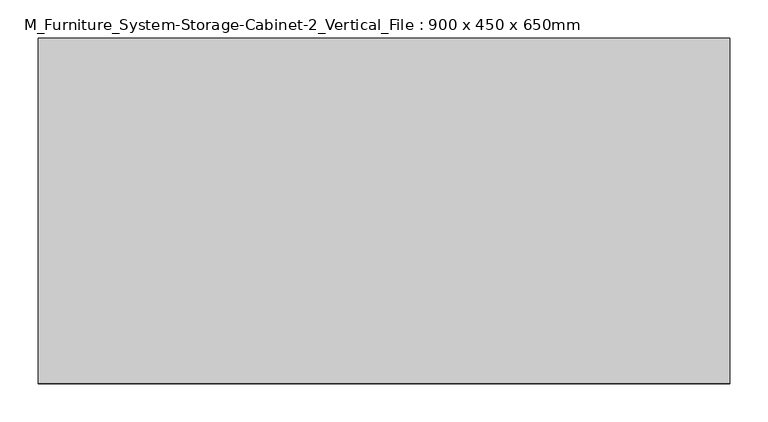
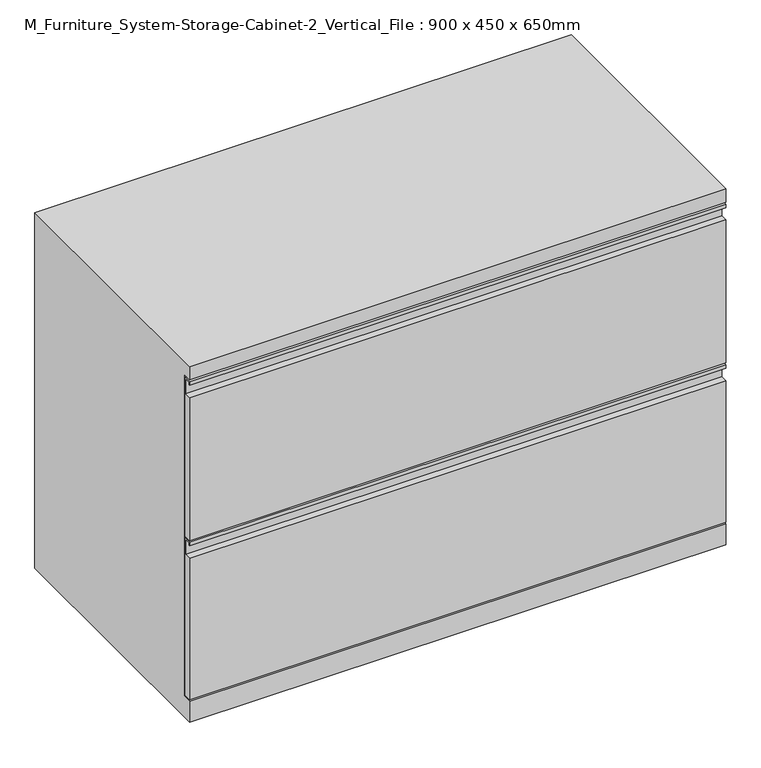
"""IFC4 building model written with IfcOpenShell, lengths in millimetres: furniture geometry, M_Furniture_System-Storage-Cabinet-2_Vertical_File : 900 x 450 x 650mm."""

from ifc_helpers import new_model, si_unit, frame, origin, place, context, project, spatial, polyline, outline, extrude, source, transform, mapped, element, save


def m_furniture_system_storage_cabinet_2_vertical_file_900_x_450_def3fd80(model_context):
    return source(origin(), model_context, "Body", "SweptSolid", [
        extrude(outline(polyline([(0.0, 341.2718803), (0.0, 594.8451302), (11.8998876, 594.8451302), (11.8998876, 621.4884893), (1.5239879, 621.4884893), (1.5239879, 616.6625121), (0.0, 616.6625121), (0.0, 623.0124879), (13.4873883, 623.0124879), (13.4873883, 341.2718803), (0.0, 341.2718803)])), frame((-450.0, 0.0, 0.0), z_axis=(1.0, 0.0, 0.0), x_axis=(0.0, 1.0, 0.0)), (0.0, 0.0, 1.0), 900.0),
        extrude(outline(polyline([(0.0, 58.7374985), (0.0, 309.9295347), (11.9293774, 309.9295347), (11.9293774, 336.5728939), (1.5239879, 336.5728939), (1.5239879, 331.7468803), (0.0, 331.7468803), (0.0, 338.0968924), (13.4873883, 338.0968924), (13.4873883, 58.7374985), (0.0, 58.7374985)])), frame((-450.0, 0.0, 0.0), z_axis=(1.0, 0.0, 0.0), x_axis=(0.0, 1.0, 0.0)), (0.0, 0.0, 1.0), 900.0),
        extrude(outline(polyline([(56.820048, 9.2063177), (51.9174039, 19.05), (100.4825718, 19.05), (95.5799278, 9.2063177), (86.9277397, 2.4185626), (76.1999879, 0.0), (65.4722406, 2.4185626), (56.820048, 9.2063177)])), frame((-396.025, 0.0, 0.0), z_axis=(1.0, 0.0, 0.0), x_axis=(0.0, 1.0, 0.0)), (0.0, 0.0, 1.0), 44.45),
        extrude(outline(polyline([(354.4200601, 9.2063177), (349.517416, 19.05), (398.082584, 19.05), (393.1799399, 9.2063177), (384.5277518, 2.4185626), (373.8, 0.0), (363.0722527, 2.4185626), (354.4200601, 9.2063177)])), frame((-396.025, 0.0, 0.0), z_axis=(1.0, 0.0, 0.0), x_axis=(0.0, 1.0, 0.0)), (0.0, 0.0, 1.0), 44.45),
        extrude(outline(polyline([(56.820048, 9.2063177), (51.9174039, 19.05), (100.4825718, 19.05), (95.5799278, 9.2063177), (86.9277397, 2.4185626), (76.1999879, 0.0), (65.4722406, 2.4185626), (56.820048, 9.2063177)])), frame((351.575, 0.0, 0.0), z_axis=(1.0, 0.0, 0.0), x_axis=(0.0, 1.0, 0.0)), (0.0, 0.0, 1.0), 44.45),
        extrude(outline(polyline([(398.082584, 19.05), (393.1799399, 9.2063177), (384.5277518, 2.4185626), (373.8, 0.0), (363.0722527, 2.4185626), (354.4200601, 9.2063177), (349.517416, 19.05), (398.082584, 19.05)])), frame((351.575, 0.0, 0.0), z_axis=(1.0, 0.0, 0.0), x_axis=(0.0, 1.0, 0.0)), (0.0, 0.0, 1.0), 44.45),
        extrude(outline(polyline([(0.0, 650.0), (450.0, 650.0), (450.0, 19.05), (0.0, 19.05), (0.0, 56.3562485), (16.6623883, 56.3562485), (16.6623883, 626.1875121), (0.0, 626.1875121), (0.0, 650.0)])), frame((-450.0, 0.0, 0.0), z_axis=(1.0, 0.0, 0.0), x_axis=(0.0, 1.0, 0.0)), (0.0, 0.0, 1.0), 900.0),
    ])


if __name__ == "__main__":
    model = new_model("IFC4")
    model_context = context("Model", 3, world=origin())
    ifc_project = project(units=[si_unit("LENGTHUNIT", "METRE", prefix="MILLI")], contexts=[model_context])
    site = spatial("IfcSite", under=ifc_project)
    building = spatial("IfcBuilding", under=site)
    placement = place(None, origin())
    m_furniture_system_storage_cabinet_2_vertical_file_900_x_450_shape = m_furniture_system_storage_cabinet_2_vertical_file_900_x_450_def3fd80(model_context)
    element("IfcFurniture", 1, ObjectType="M_Furniture_System-Storage-Cabinet-2_Vertical_File : 900 x 450 x 650mm", at=placement, inside=building, context=model_context, shape_type="MappedRepresentation", body=[
        mapped(m_furniture_system_storage_cabinet_2_vertical_file_900_x_450_shape, transform((0.0, 0.0, 0.0), x_axis=(1.0, 0.0, 0.0), y_axis=(0.0, 1.0, 0.0), z_axis=(0.0, 0.0, 1.0))),
    ])
    save(model, "model.ifc")

# Revit data of these elements
# Type "M_Furniture_System-Storage-Cabinet-2_Vertical_File : 900 x 450 x 650mm"
#   Type Comments = "900 x 450 x 650mm Double Vertical File Cabinet"
#   Width = 900 mm
#   Height = 650 mm
#   Depth = 450 mm
#   Show Solid [instance default] = yes
#   Show Dashed [instance default] = no
#   Drawer Finish [instance default] = Metal - Paint - Beige
#   Cabinet Material [instance default] = Metal - Paint - Beige
#   Model = ""
#   Manufacturer = ""
#   Description = (empty or 0)
#   Default Elevation = 0
# Element 1 (IfcFurniture, "M_Furniture_System-Storage-Cabinet-2_Vertical_File : 900 x 450 x 650mm")
#   Materials on its faces: "Metal - Paint - Beige"
# Materials
#   "Metal - Paint - Beige": class "Metal", colour RGB 247 225 182, transparency 0
